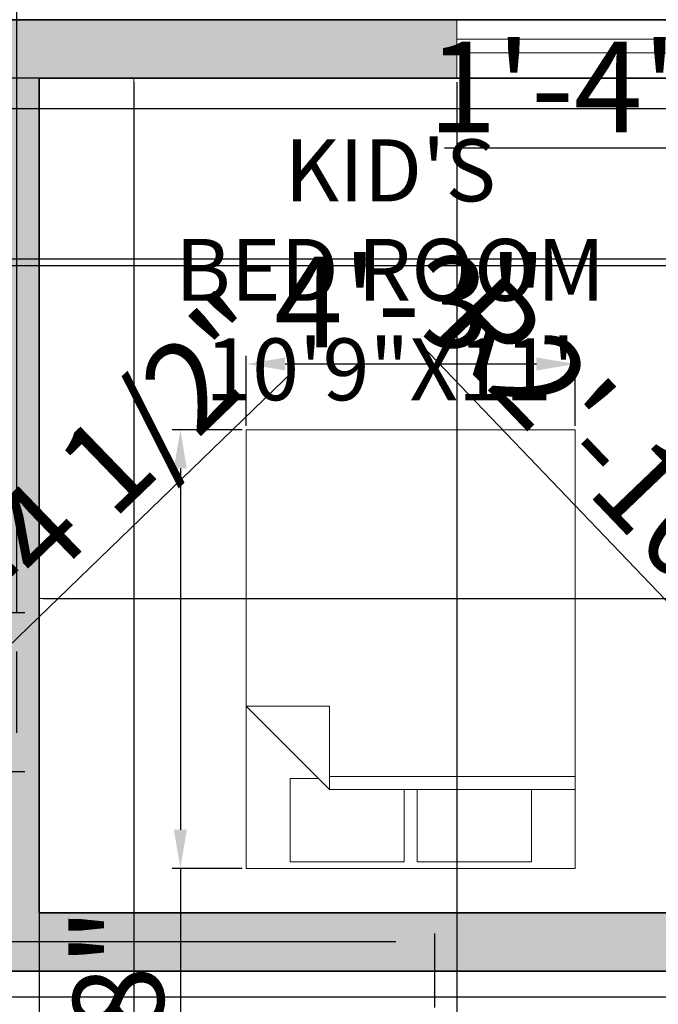
# Model space of a CAD drawing. Units: inches. Extents: x 2961 to 3748, y 1432 to 1961.
# Tile 5 of 9: x 3120 to 3219, y 1713 to 1865. Entities that reach past the tile are written whole.
import ezdxf
from ezdxf.enums import TextEntityAlignment as Align

# ---------------------------------------------------------------- set-up
doc = ezdxf.new("R2010")
doc.units = ezdxf.units.IN
for name, color, linetype, lineweight in [('A-ANNO-DIMS', 2, 'Continuous', 18), ('A-AREA-IDEN', 7, 'Continuous', 18), ('A-FURN', 8, 'Continuous', 18), ('A-FURN-FIXD', 9, 'Continuous', 20), ('A-GLAZ', 4, 'Continuous', 18), ('A-WALL', 7, 'Continuous', 35), ('A-WALL-PATT', 252, 'Continuous', 13)]:
    doc.layers.add(name, color=color, linetype=linetype, lineweight=lineweight)
doc.styles.get("Standard").update_dxf_attribs({"font": 'arial.ttf'})
doc.dimstyles.new('ISO-25', dxfattribs={"dimtxt": 14, "dimasz": 6, "dimexe": 1.25, "dimexo": 0.625, "dimtad": 1, "dimlunit": 3, "dimtxsty": 'Standard', "dimcen": 2.5, "dimadec": 0, "dimazin": 0, "dimtfac": 1, "dimtmove": 0, "dimatfit": 3, "dimfxl": 1, "dimarcsym": 0})

# ---------------------------------------------------------------- blocks, each defined once
blk = doc.blocks.new('Bed - Queen')
for p, q in [((0, -80.00003), (0, 0)), ((0, 0), (59.99999, 0)), ((59.99999, 0), (59.99999, -80.00003)), ((7.99999, -1.2), (28.79998, -1.2)), ((7.99999, -14.4), (7.99999, -1.2)), ((28.79998, -1.2), (28.79998, -14.4)), ((31.19999, -1.2), (51.99999, -1.2)), ((31.19999, -14.4), (31.19999, -1.2)), ((51.99999, -1.2), (51.99999, -16.4)), ((0, -14.4), (44.8, -14.4)), ((59.99999, -29.6), (44.8, -14.4)), ((44.8, -14.4), (44.8, -29.6)), ((44.8, -16.8), (0, -16.8)), ((51.99999, -16.4), (46.79936, -16.4)), ((44.8, -29.6), (59.99999, -29.6)), ((59.99999, -80.00003), (0, -80.00003))]:
    blk.add_line(p, q)
blk = doc.blocks.new('*D14')
at = {"layer": 'A-ANNO-DIMS', "color": 0, "lineweight": -2, "transparency": 16777216}
for p, q in [((3054.27, 1865.26), (3054.27, 1895.31)), ((3603.27, 1865.26), (3603.27, 1895.31)), ((3060.27, 1894.06), (3597.27, 1894.06))]:
    blk.add_line(p, q, dxfattribs=at)
at = {"layer": 'A-ANNO-DIMS', "color": 0, "transparency": 16777216}
for points in [[(3060.27, 1895.06), (3060.27, 1893.06), (3054.27, 1894.06)], [(3597.27, 1895.06), (3597.27, 1893.06), (3603.27, 1894.06)]]:
    blk.add_solid(points, dxfattribs=at)
at = {"layer": 'Defpoints', "color": 0, "transparency": 16777216}
for p in [(3603.27, 1894.06), (3054.27, 1864.64), (3603.27, 1864.64)]:
    blk.add_point(p, dxfattribs=at)
at = {"layer": 'A-ANNO-DIMS', "color": 0, "transparency": 16777216, "insert": (3328.77, 1901.84), "char_height": 14, "attachment_point": 5}
blk.add_mtext('45\'-9"', dxfattribs=at)
blk = doc.blocks.new('WIN-36IN')
for p, q in [((0, 6), (36, 6)), ((0, 3.9), (36, 3.9))]:
    blk.add_line(p, q)
blk.add_lwpolyline([(36, 9), (0, 9), (0, 0), (36, 0)], close=True)
blk = doc.blocks.new('*D24')
at = {"layer": 'A-ANNO-DIMS', "color": 0, "lineweight": -2, "transparency": 16777216}
for p, q in [((3154.63, 1801.29), (3143.84, 1801.29)), ((3145.09, 1795.29), (3145.09, 1739.5)), ((3154.63, 1733.5), (3143.84, 1733.5)), ((3145.09, 1733.5), (3145.09, 1644.01))]:
    blk.add_line(p, q, dxfattribs=at)
at = {"layer": 'A-ANNO-DIMS', "color": 0, "transparency": 16777216}
for points in [[(3144.09, 1795.29), (3146.09, 1795.29), (3145.09, 1801.29)], [(3144.09, 1739.5), (3146.09, 1739.5), (3145.09, 1733.5)]]:
    blk.add_solid(points, dxfattribs=at)
at = {"layer": 'Defpoints', "color": 0, "transparency": 16777216}
for p in [(3155.26, 1801.29), (3145.09, 1733.5), (3155.26, 1733.5)]:
    blk.add_point(p, dxfattribs=at)
at = {"layer": 'A-ANNO-DIMS', "color": 0, "transparency": 16777216, "insert": (3137.32, 1685.76), "char_height": 14, "attachment_point": 5, "rotation": 90}
blk.add_mtext('BED 5\'-8"', dxfattribs=at)
blk = doc.blocks.new('*D25')
at = {"layer": 'A-ANNO-DIMS', "color": 0, "lineweight": -2, "transparency": 16777216}
for p, q in [((3155.26, 1801.92), (3155.26, 1812.71)), ((3206.1, 1801.92), (3206.1, 1812.71)), ((3200.1, 1811.46), (3161.26, 1811.46))]:
    blk.add_line(p, q, dxfattribs=at)
at = {"layer": 'A-ANNO-DIMS', "color": 0, "transparency": 16777216}
for points in [[(3161.26, 1812.46), (3161.26, 1810.46), (3155.26, 1811.46)], [(3200.1, 1812.46), (3200.1, 1810.46), (3206.1, 1811.46)]]:
    blk.add_solid(points, dxfattribs=at)
at = {"layer": 'Defpoints', "color": 0, "transparency": 16777216}
for p in [(3155.26, 1811.46), (3155.26, 1801.29), (3206.1, 1801.29)]:
    blk.add_point(p, dxfattribs=at)
at = {"layer": 'A-ANNO-DIMS', "color": 0, "transparency": 16777216, "insert": (3180.68, 1819.24), "char_height": 14, "attachment_point": 5}
blk.add_mtext('4\'-3"', dxfattribs=at)
blk = doc.blocks.new('*D26')
at = {"layer": 'A-ANNO-DIMS', "color": 0, "lineweight": -2, "transparency": 16777216}
for p, q in [((3112.4, 1712.02), (3112.4, 1723.44)), ((3184.4, 1712.02), (3184.4, 1723.44)), ((3112.4, 1722.19), (2961.2, 1722.19)), ((3178.4, 1722.19), (3118.4, 1722.19))]:
    blk.add_line(p, q, dxfattribs=at)
at = {"layer": 'A-ANNO-DIMS', "color": 0, "transparency": 16777216}
for points in [[(3118.4, 1723.19), (3118.4, 1721.19), (3112.4, 1722.19)], [(3178.4, 1723.19), (3178.4, 1721.19), (3184.4, 1722.19)]]:
    blk.add_solid(points, dxfattribs=at)
at = {"layer": 'Defpoints', "color": 0, "transparency": 16777216}
for p in [(3112.4, 1722.19), (3112.4, 1711.39), (3184.4, 1711.39)]:
    blk.add_point(p, dxfattribs=at)
at = {"layer": 'A-ANNO-DIMS', "color": 0, "transparency": 16777216, "insert": (3033.8, 1730.06), "char_height": 14, "attachment_point": 5}
blk.add_mtext('SOFA 6\'-0" TYP.', dxfattribs=at)
blk = doc.blocks.new('*D28')
at = {"layer": 'A-ANNO-DIMS', "color": 0, "lineweight": -2, "transparency": 16777216}
for p, q in [((3253.06, 1631.67), (3253.06, 1776.5)), ((3245.67, 1631.67), (3254.31, 1631.67)), ((3253.06, 1584.22), (3253.06, 1625.67)), ((3245.67, 1578.22), (3254.31, 1578.22))]:
    blk.add_line(p, q, dxfattribs=at)
at = {"layer": 'A-ANNO-DIMS', "color": 0, "transparency": 16777216}
for points in [[(3252.06, 1625.67), (3254.06, 1625.67), (3253.06, 1631.67)], [(3252.06, 1584.22), (3254.06, 1584.22), (3253.06, 1578.22)]]:
    blk.add_solid(points, dxfattribs=at)
at = {"layer": 'Defpoints', "color": 0, "transparency": 16777216}
for p in [(3245.04, 1631.67), (3253.06, 1631.67), (3245.04, 1578.22)]:
    blk.add_point(p, dxfattribs=at)
at = {"layer": 'A-ANNO-DIMS', "color": 0, "transparency": 16777216, "insert": (3245.19, 1707.08), "char_height": 14, "attachment_point": 5, "rotation": 90}
blk.add_mtext('TABLE 4\'-5 1/2"', dxfattribs=at)
blk = doc.blocks.new('*D31')
at = {"layer": 'A-ANNO-DIMS', "color": 0, "lineweight": -2, "transparency": 16777216}
for p, q in [((3229.02, 1840.61), (3229.02, 1846.04)), ((3245.04, 1840.61), (3245.04, 1846.04)), ((3229.02, 1844.79), (3185.88, 1844.79)), ((3239.04, 1844.79), (3235.02, 1844.79))]:
    blk.add_line(p, q, dxfattribs=at)
at = {"layer": 'A-ANNO-DIMS', "color": 0, "transparency": 16777216}
for points in [[(3235.02, 1845.79), (3235.02, 1843.79), (3229.02, 1844.79)], [(3239.04, 1845.79), (3239.04, 1843.79), (3245.04, 1844.79)]]:
    blk.add_solid(points, dxfattribs=at)
at = {"layer": 'Defpoints', "color": 0, "transparency": 16777216}
for p in [(3229.02, 1844.79), (3229.02, 1839.99), (3245.04, 1839.99)]:
    blk.add_point(p, dxfattribs=at)
at = {"layer": 'A-ANNO-DIMS', "color": 0, "transparency": 16777216, "insert": (3204.45, 1852.45), "char_height": 14, "attachment_point": 5}
blk.add_mtext('1\'-4"', dxfattribs=at)
blk = doc.blocks.new('*D46')
at = {"layer": 'A-ANNO-DIMS', "color": 0, "lineweight": -2, "transparency": 16777216}
for p, q in [((3119.82, 1773.04), (3119.82, 1913.63)), ((3116.76, 1773.04), (3121.07, 1773.04)), ((3119.82, 1754.49), (3119.82, 1767.04)), ((3116.76, 1748.49), (3121.07, 1748.49))]:
    blk.add_line(p, q, dxfattribs=at)
at = {"layer": 'A-ANNO-DIMS', "color": 0, "transparency": 16777216}
for points in [[(3118.82, 1767.04), (3120.82, 1767.04), (3119.82, 1773.04)], [(3118.82, 1754.49), (3120.82, 1754.49), (3119.82, 1748.49)]]:
    blk.add_solid(points, dxfattribs=at)
at = {"layer": 'Defpoints', "color": 0, "transparency": 16777216}
for p in [(3116.13, 1773.04), (3119.82, 1773.04), (3116.13, 1748.49)]:
    blk.add_point(p, dxfattribs=at)
at = {"layer": 'A-ANNO-DIMS', "color": 0, "transparency": 16777216, "insert": (3111.95, 1846.34), "char_height": 14, "attachment_point": 5, "rotation": 90}
blk.add_mtext('BASIN 2\'-0 1/2"', dxfattribs=at)
blk = doc.blocks.new('*D53')
at = {"layer": 'A-ANNO-DIMS', "color": 0, "lineweight": -2, "transparency": 16777216}
for p, q in [((3123.27, 1855.01), (3123.27, 1473.94)), ((3187.8, 1855.01), (3187.8, 1473.94)), ((3129.27, 1475.19), (3181.8, 1475.19)), ((3187.8, 1475.19), (3264.89, 1475.19))]:
    blk.add_line(p, q, dxfattribs=at)
at = {"layer": 'A-ANNO-DIMS', "color": 0, "transparency": 16777216}
for points in [[(3129.27, 1476.19), (3129.27, 1474.19), (3123.27, 1475.19)], [(3181.8, 1476.19), (3181.8, 1474.19), (3187.8, 1475.19)]]:
    blk.add_solid(points, dxfattribs=at)
at = {"layer": 'Defpoints', "color": 0, "transparency": 16777216}
for p in [(3123.27, 1855.64), (3187.8, 1855.64), (3187.8, 1475.19)]:
    blk.add_point(p, dxfattribs=at)
at = {"layer": 'A-ANNO-DIMS', "color": 0, "transparency": 16777216, "insert": (3229.35, 1483.05), "char_height": 14, "attachment_point": 5}
blk.add_mtext('5\'-4 1/2"', dxfattribs=at)
blk = doc.blocks.new('*D64')
at = {"layer": 'A-ANNO-DIMS', "color": 0, "lineweight": -2, "transparency": 16777216}
for p, q in [((3509.64, 1855.64), (3023.57, 1855.64)), ((3024.82, 1849.64), (3024.82, 1833.64)), ((3509.64, 1827.64), (3023.57, 1827.64)), ((3024.82, 1827.64), (3024.82, 1782.93))]:
    blk.add_line(p, q, dxfattribs=at)
at = {"layer": 'A-ANNO-DIMS', "color": 0, "transparency": 16777216}
for points in [[(3023.82, 1849.64), (3025.82, 1849.64), (3024.82, 1855.64)], [(3023.82, 1833.64), (3025.82, 1833.64), (3024.82, 1827.64)]]:
    blk.add_solid(points, dxfattribs=at)
at = {"layer": 'Defpoints', "color": 0, "transparency": 16777216}
for p in [(3510.27, 1855.64), (3024.82, 1827.64), (3510.27, 1827.64)]:
    blk.add_point(p, dxfattribs=at)
at = {"layer": 'A-ANNO-DIMS', "color": 0, "transparency": 16777216, "insert": (3017.16, 1802.29), "char_height": 14, "attachment_point": 5, "rotation": 90}
blk.add_mtext('2\'-4"', dxfattribs=at)
blk = doc.blocks.new('*D73')
at = {"layer": 'A-ANNO-DIMS', "color": 0, "lineweight": -2, "transparency": 16777216}
for p, q in [((3069.27, 1717.01), (3069.27, 1473.94)), ((3103.27, 1717.01), (3103.27, 1473.94)), ((3075.27, 1475.19), (3097.27, 1475.19)), ((3103.27, 1475.19), (3158.85, 1475.19))]:
    blk.add_line(p, q, dxfattribs=at)
at = {"layer": 'A-ANNO-DIMS', "color": 0, "transparency": 16777216}
for points in [[(3075.27, 1476.19), (3075.27, 1474.19), (3069.27, 1475.19)], [(3097.27, 1476.19), (3097.27, 1474.19), (3103.27, 1475.19)]]:
    blk.add_solid(points, dxfattribs=at)
at = {"layer": 'Defpoints', "color": 0, "transparency": 16777216}
for p in [(3069.27, 1717.64), (3103.27, 1717.64), (3103.27, 1475.19)]:
    blk.add_point(p, dxfattribs=at)
at = {"layer": 'A-ANNO-DIMS', "color": 0, "transparency": 16777216, "insert": (3134.06, 1482.96), "char_height": 14, "attachment_point": 5}
blk.add_mtext('2\'-10"', dxfattribs=at)
blk = doc.blocks.new('*D74')
at = {"layer": 'A-ANNO-DIMS', "color": 0, "lineweight": -2, "transparency": 16777216}
for p, q in [((3117.27, 1726.01), (3117.27, 1473.94)), ((3103.27, 1717.01), (3103.27, 1473.94)), ((3109.27, 1475.19), (3111.27, 1475.19)), ((3117.27, 1475.19), (3160.41, 1475.19))]:
    blk.add_line(p, q, dxfattribs=at)
at = {"layer": 'A-ANNO-DIMS', "color": 0, "transparency": 16777216}
for points in [[(3109.27, 1476.19), (3109.27, 1474.19), (3103.27, 1475.19)], [(3111.27, 1476.19), (3111.27, 1474.19), (3117.27, 1475.19)]]:
    blk.add_solid(points, dxfattribs=at)
at = {"layer": 'Defpoints', "color": 0, "transparency": 16777216}
for p in [(3117.27, 1726.64), (3103.27, 1717.64), (3117.27, 1475.19)]:
    blk.add_point(p, dxfattribs=at)
at = {"layer": 'A-ANNO-DIMS', "color": 0, "transparency": 16777216, "insert": (3141.84, 1482.84), "char_height": 14, "attachment_point": 5}
blk.add_mtext('1\'-2"', dxfattribs=at)
blk = doc.blocks.new('*D75')
at = {"layer": 'A-ANNO-DIMS', "color": 0, "lineweight": -2, "transparency": 16777216}
for p, q in [((3024.82, 1723.64), (3024.82, 1729.64)), ((3254.64, 1717.64), (3023.57, 1717.64)), ((3024.82, 1717.64), (3024.82, 1713.64)), ((3254.64, 1713.64), (3023.57, 1713.64)), ((3024.82, 1707.64), (3024.82, 1663.17))]:
    blk.add_line(p, q, dxfattribs=at)
at = {"layer": 'A-ANNO-DIMS', "color": 0, "transparency": 16777216}
for points in [[(3023.82, 1723.64), (3025.82, 1723.64), (3024.82, 1717.64)], [(3023.82, 1707.64), (3025.82, 1707.64), (3024.82, 1713.64)]]:
    blk.add_solid(points, dxfattribs=at)
at = {"layer": 'Defpoints', "color": 0, "transparency": 16777216}
for p in [(3255.27, 1717.64), (3024.82, 1713.64), (3255.27, 1713.64)]:
    blk.add_point(p, dxfattribs=at)
at = {"layer": 'A-ANNO-DIMS', "color": 0, "transparency": 16777216, "insert": (3017.04, 1682.41), "char_height": 14, "attachment_point": 5, "rotation": 90}
blk.add_mtext('0\'-4"', dxfattribs=at)
blk = doc.blocks.new('*D82')
at = {"layer": 'A-ANNO-DIMS', "color": 0, "lineweight": -2, "transparency": 16777216}
for p, q in [((3063.27, 1542.49), (3063.27, 1933.63)), ((3069.27, 1932.38), (3078.82, 1932.38)), ((3084.82, 1542.49), (3084.82, 1933.63)), ((3084.82, 1932.38), (3160.59, 1932.38))]:
    blk.add_line(p, q, dxfattribs=at)
at = {"layer": 'A-ANNO-DIMS', "color": 0, "transparency": 16777216}
for points in [[(3069.27, 1933.38), (3069.27, 1931.38), (3063.27, 1932.38)], [(3078.82, 1933.38), (3078.82, 1931.38), (3084.82, 1932.38)]]:
    blk.add_solid(points, dxfattribs=at)
at = {"layer": 'Defpoints', "color": 0, "transparency": 16777216}
for p in [(3084.82, 1932.38), (3063.27, 1541.87), (3084.82, 1541.87)]:
    blk.add_point(p, dxfattribs=at)
at = {"layer": 'A-ANNO-DIMS', "color": 0, "transparency": 16777216, "insert": (3125.71, 1940.24), "char_height": 14, "attachment_point": 5}
blk.add_mtext('1\'-9 1/2"', dxfattribs=at)
blk = doc.blocks.new('*D83')
at = {"layer": 'A-ANNO-DIMS', "color": 0, "lineweight": -2, "transparency": 16777216}
for p, q in [((3123.89, 1855.64), (3633.97, 1855.64)), ((3632.72, 1781.22), (3632.72, 1849.64)), ((3123.89, 1775.22), (3633.97, 1775.22))]:
    blk.add_line(p, q, dxfattribs=at)
at = {"layer": 'A-ANNO-DIMS', "color": 0, "transparency": 16777216}
for points in [[(3631.72, 1849.64), (3633.72, 1849.64), (3632.72, 1855.64)], [(3631.72, 1781.22), (3633.72, 1781.22), (3632.72, 1775.22)]]:
    blk.add_solid(points, dxfattribs=at)
at = {"layer": 'Defpoints', "color": 0, "transparency": 16777216}
for p in [(3123.27, 1855.64), (3632.72, 1855.64), (3123.27, 1775.22)]:
    blk.add_point(p, dxfattribs=at)
at = {"layer": 'A-ANNO-DIMS', "color": 0, "transparency": 16777216, "insert": (3624.85, 1815.43), "char_height": 14, "attachment_point": 5, "rotation": 90}
blk.add_mtext('6\'-8 1/2"', dxfattribs=at)
blk = doc.blocks.new('*D84')
at = {"layer": 'A-ANNO-DIMS', "color": 0, "lineweight": -2, "transparency": 16777216}
for p, q in [((3123.27, 1855.01), (3123.27, 1473.94)), ((3137.88, 1855.01), (3137.88, 1473.94)), ((3129.27, 1475.19), (3131.88, 1475.19)), ((3137.88, 1475.19), (3213.65, 1475.19))]:
    blk.add_line(p, q, dxfattribs=at)
at = {"layer": 'A-ANNO-DIMS', "color": 0, "transparency": 16777216}
for points in [[(3129.27, 1476.19), (3129.27, 1474.19), (3123.27, 1475.19)], [(3131.88, 1476.19), (3131.88, 1474.19), (3137.88, 1475.19)]]:
    blk.add_solid(points, dxfattribs=at)
at = {"layer": 'Defpoints', "color": 0, "transparency": 16777216}
for p in [(3123.27, 1855.64), (3137.88, 1855.64), (3137.88, 1475.19)]:
    blk.add_point(p, dxfattribs=at)
at = {"layer": 'A-ANNO-DIMS', "color": 0, "transparency": 16777216, "insert": (3178.76, 1483.05), "char_height": 14, "attachment_point": 5}
blk.add_mtext('1\'-2 1/2"', dxfattribs=at)
blk = doc.blocks.new('*D86')
at = {"layer": 'A-ANNO-DIMS', "color": 0, "lineweight": -2, "transparency": 16777216}
for p, q in [((3091.52, 1850.93), (3633.97, 1850.93)), ((3632.72, 1844.93), (3632.72, 1832.66)), ((3082.42, 1826.66), (3633.97, 1826.66)), ((3632.72, 1826.66), (3632.72, 1749.34))]:
    blk.add_line(p, q, dxfattribs=at)
at = {"layer": 'A-ANNO-DIMS', "color": 0, "transparency": 16777216}
for points in [[(3631.72, 1844.93), (3633.72, 1844.93), (3632.72, 1850.93)], [(3631.72, 1832.66), (3633.72, 1832.66), (3632.72, 1826.66)]]:
    blk.add_solid(points, dxfattribs=at)
at = {"layer": 'Defpoints', "color": 0, "transparency": 16777216}
for p in [(3090.9, 1850.93), (3081.8, 1826.66), (3632.72, 1826.66)]:
    blk.add_point(p, dxfattribs=at)
at = {"layer": 'A-ANNO-DIMS', "color": 0, "transparency": 16777216, "insert": (3624.85, 1785), "char_height": 14, "attachment_point": 5, "rotation": 90}
blk.add_mtext('2\'-0 1/2"', dxfattribs=at)
blk = doc.blocks.new('*D94')
at = {"layer": 'A-ANNO-DIMS', "color": 0, "lineweight": -2, "transparency": 16777216}
for p, q in [((3182.5, 1814.2), (3230.05, 1764.56)), ((3257.56, 1735.84), (3234.2, 1760.22))]:
    blk.add_line(p, q, dxfattribs=at)
at = {"layer": 'A-ANNO-DIMS', "color": 0, "transparency": 16777216}
blk.add_solid([(3230.78, 1765.25), (3229.33, 1763.87), (3234.2, 1760.22)], dxfattribs=at)
at = {"layer": 'Defpoints', "color": 0, "transparency": 16777216}
for p in [(3234.2, 1760.22), (3257.56, 1735.84)]:
    blk.add_point(p, dxfattribs=at)
at = {"layer": 'A-ANNO-DIMS', "color": 0, "transparency": 16777216, "insert": (3209.82, 1796.92), "char_height": 14, "attachment_point": 5, "rotation": 313.7658}
blk.add_mtext('R2\'-10"', dxfattribs=at)
blk = doc.blocks.new('*D95')
at = {"layer": 'A-ANNO-DIMS', "color": 0, "lineweight": -2, "transparency": 16777216}
for p, q in [((3162.66, 1810.5), (3097.6, 1747.61)), ((3072.77, 1723.61), (3093.28, 1743.44))]:
    blk.add_line(p, q, dxfattribs=at)
at = {"layer": 'A-ANNO-DIMS', "color": 0, "transparency": 16777216}
blk.add_solid([(3096.9, 1748.33), (3098.29, 1746.89), (3093.28, 1743.44)], dxfattribs=at)
at = {"layer": 'Defpoints', "color": 0, "transparency": 16777216}
for p in [(3093.28, 1743.44), (3072.77, 1723.61)]:
    blk.add_point(p, dxfattribs=at)
at = {"layer": 'A-ANNO-DIMS', "color": 0, "transparency": 16777216, "insert": (3126.82, 1786.79), "char_height": 14, "attachment_point": 5, "rotation": 44.0296}
blk.add_mtext('R2\'-4 1/2"', dxfattribs=at)

msp = doc.modelspace()

# ---------------------------------------------------------------- hatches: boundary and pattern name
at = {"layer": 'A-WALL-PATT'}
h = msp.add_hatch(color=256, dxfattribs=at)
h.set_gradient(color1=(41, 49, 137), color2=(41, 49, 137), tint=1)
h.paths.add_polyline_path([(3255.267, 1671.639), (3255.267, 1513.639), (3251.267, 1513.639), (3251.267, 1504.639), (3268.267, 1504.639), (3268.267, 1513.639), (3264.267, 1513.639), (3264.267, 1671.639), (3259.767, 1671.639)])
h.paths.add_polyline_path([(3063.267, 1513.639), (3063.267, 1677.639), (3054.267, 1677.639), (3054.267, 1504.639), (3215.267, 1504.639), (3215.267, 1513.639)])
h.paths.add_polyline_path([(3304.267, 1513.639), (3304.267, 1504.639), (3456.267, 1504.639), (3456.267, 1513.639), (3390.267, 1513.639), (3390.267, 1605.639), (3384.267, 1605.639), (3384.267, 1513.639)])
h.paths.add_polyline_path([(3510.267, 1605.639), (3510.267, 1513.639), (3492.267, 1513.639), (3492.267, 1504.639), (3546.267, 1504.639), (3546.267, 1513.639), (3519.267, 1513.639), (3519.267, 1605.639)])
h.paths.add_polyline_path([(3340.267, 1654.639), (3340.267, 1645.639), (3510.267, 1645.639), (3510.267, 1641.639), (3519.267, 1641.639), (3519.267, 1658.639), (3510.267, 1658.639), (3510.267, 1654.639)])
h.paths.add_polyline_path([(3223.801, 1864.639), (3223.801, 1855.639), (3255.267, 1855.639), (3255.267, 1772.534), (3264.267, 1772.534), (3264.267, 1855.639), (3303.267, 1855.639), (3303.267, 1864.639)])
h.paths.add_polyline_path([(3339.267, 1864.639), (3339.267, 1855.639), (3435.267, 1855.639), (3435.267, 1864.639)])
h.paths.add_polyline_path([(3471.267, 1864.639), (3471.267, 1855.639), (3510.267, 1855.639), (3510.267, 1827.639), (3519.267, 1827.639), (3519.267, 1864.639)])
h.paths.add_polyline_path([(3510.267, 1767.639), (3510.267, 1739.639), (3519.267, 1739.639), (3519.267, 1767.639)])
h.paths.add_polyline_path([(3123.267, 1726.639), (3123.267, 1855.639), (3187.801, 1855.639), (3187.801, 1864.639), (3054.267, 1864.639), (3054.267, 1837.201), (3063.267, 1837.201), (3063.267, 1855.639), (3117.267, 1855.639), (3117.267, 1726.639), (3103.267, 1726.639), (3103.267, 1717.639), (3255.267, 1717.639), (3255.267, 1713.639), (3264.267, 1713.639), (3264.267, 1730.534), (3255.267, 1730.639), (3255.267, 1726.639)])
h.paths.add_polyline_path([(3597.267, 1654.639), (3597.267, 1513.639), (3570.267, 1513.639), (3570.267, 1504.639), (3603.267, 1504.639), (3603.267, 1654.639)])
h.paths.add_polyline_path([(3054.267, 1813.201), (3054.267, 1713.639), (3063.267, 1713.639), (3063.267, 1717.639), (3069.267, 1717.639), (3069.267, 1726.639), (3063.267, 1726.639), (3063.267, 1813.201)], flags=17)

# ---------------------------------------------------------------- linework, layer by layer
at = {"layer": 'A-FURN-FIXD'}
msp.add_lwpolyline([(3123.267, 1775.22), (3123.267, 1855.639), (3137.877, 1855.639), (3137.877, 1775.22)], close=True, dxfattribs=at)
at = {"layer": 'A-WALL'}
for p, q in [((3054.267, 1864.639), (3519.267, 1864.639)), ((3123.267, 1726.639), (3123.267, 1855.639)), ((3255.267, 1855.639), (3123.267, 1855.639)), ((3255.267, 1726.639), (3123.267, 1726.639)), ((3255.267, 1717.639), (3063.267, 1717.639))]:
    msp.add_line(p, q, dxfattribs=at)

# ---------------------------------------------------------------- block references
at = {"layer": 'A-FURN', "xscale": 0.8473786619107851, "yscale": 0.8473786619107851, "zscale": 0.8473786619107851, "rotation": 180}
msp.add_blockref('Bed - Queen', (3206.1, 1733.502), dxfattribs=at)
at = {"layer": 'A-GLAZ'}
msp.add_blockref('WIN-36IN', (3187.801, 1855.639), dxfattribs=at)

# ---------------------------------------------------------------- texts
at = {"layer": 'A-AREA-IDEN'}
for s, p in [("KID'S", (3177.513, 1836.597)), ('BED ROOM', (3177.513, 1821.223)), ('10\'9"X11\'', (3177.513, 1805.848))]:
    msp.add_text(s, height=9.5707, dxfattribs=at).set_placement(p, align=Align.CENTER)

# ---------------------------------------------------------------- dimensions: what is measured, and where the dimension line sits
at = {"layer": 'A-ANNO-DIMS'}
for base, p1, p2, override, picture, middle in [((3084.825, 1932.38), (3063.267, 1541.867), (3084.825, 1541.867), {"dimdec": 1, "dimlfac": 1, "dimrnd": 0, "dimzin": 1, "dimdsep": 46, "dimlunit": 4, "dimfrac": 2}, '*D82', (3125.71, 1940.244)), ((3603.267, 1894.063), (3054.267, 1864.639), (3603.267, 1864.639), {"dimclrd": 0, "dimclre": 0, "dimclrt": 0}, '*D14', (3328.767, 1901.836)), ((3187.801, 1475.189), (3123.267, 1855.639), (3187.801, 1855.639), {"dimdec": 1, "dimlfac": 1, "dimrnd": 0, "dimzin": 1, "dimdsep": 46, "dimlunit": 4, "dimfrac": 2}, '*D53', (3229.345, 1483.052)), ((3137.877, 1475.189), (3123.267, 1855.639), (3137.877, 1855.639), {"dimdec": 1, "dimlfac": 1, "dimrnd": 0, "dimzin": 1, "dimdsep": 46, "dimlunit": 4, "dimfrac": 2}, '*D84', (3178.762, 1483.052)), ((3117.267, 1475.189), (3103.267, 1717.639), (3117.267, 1726.639), {"dimdec": 1, "dimlfac": 1, "dimrnd": 0, "dimzin": 1, "dimdsep": 46, "dimlunit": 4, "dimfrac": 2}, '*D74', (3141.841, 1482.842)), ((3103.267, 1475.189), (3069.267, 1717.639), (3103.267, 1717.639), {"dimdec": 1, "dimlfac": 1, "dimrnd": 0, "dimzin": 1, "dimdsep": 46, "dimlunit": 4, "dimfrac": 2}, '*D73', (3134.058, 1482.962))]:
    dim = msp.add_linear_dim(base=base, p1=p1, p2=p2, dimstyle='ISO-25', override=override, dxfattribs=at)
    dim.commit()
    dim.dimension.update_dxf_attribs({"geometry": picture, "text_midpoint": middle})
for base, p1, p2, angle, text, picture, middle in [((3119.818, 1773.04), (3116.135, 1748.489), (3116.135, 1773.04), 90, 'BASIN <>', '*D46', (3111.954, 1846.336)), ((3145.088, 1733.502), (3155.257, 1801.293), (3155.257, 1733.502), 270, 'BED <>', '*D24', (3137.315, 1685.756)), ((3253.058, 1631.667), (3245.042, 1578.224), (3245.042, 1631.667), 90, 'TABLE <>', '*D28', (3245.195, 1707.084)), ((3112.401, 1722.191), (3184.401, 1711.391), (3112.401, 1711.391), 180, 'SOFA <> TYP.', '*D26', (3033.799, 1730.06))]:
    dim = msp.add_linear_dim(base=base, p1=p1, p2=p2, angle=angle, text=text, dimstyle='ISO-25', override={"dimdec": 1, "dimlfac": 1, "dimrnd": 0, "dimzin": 1, "dimdsep": 46, "dimlunit": 4, "dimfrac": 2}, dxfattribs=at)
    dim.commit()
    dim.dimension.update_dxf_attribs({"geometry": picture, "text_midpoint": middle})
for base, p1, p2, angle, picture, middle in [((3229.024, 1844.793), (3245.042, 1839.987), (3229.024, 1839.987), 180, '*D31', (3204.45, 1852.446)), ((3024.817, 1827.639), (3510.267, 1855.639), (3510.267, 1827.639), 90, '*D64', (3017.163, 1802.287)), ((3632.717, 1855.639), (3123.267, 1775.22), (3123.267, 1855.639), 90, '*D83', (3624.853, 1815.429)), ((3632.717, 1826.664), (3090.897, 1850.93), (3081.797, 1826.664), 90, '*D86', (3624.853, 1785)), ((3155.257, 1811.461), (3206.1, 1801.293), (3155.257, 1801.293), 180, '*D25', (3180.678, 1819.239)), ((3024.817, 1713.639), (3255.267, 1717.639), (3255.267, 1713.639), 90, '*D75', (3017.044, 1682.406))]:
    dim = msp.add_linear_dim(base=base, p1=p1, p2=p2, angle=angle, dimstyle='ISO-25', override={"dimdec": 1, "dimlfac": 1, "dimrnd": 0, "dimzin": 1, "dimdsep": 46, "dimlunit": 4, "dimfrac": 2}, dxfattribs=at)
    dim.commit()
    dim.dimension.update_dxf_attribs({"geometry": picture, "text_midpoint": middle})
for center, mpoint, picture, middle in [((3257.563, 1735.836), (3234.204, 1760.224), '*D94', (3209.817, 1796.922)), ((3072.767, 1723.605), (3093.285, 1743.44), '*D95', (3126.819, 1786.794))]:
    dim = msp.add_radius_dim(center=center, mpoint=mpoint, dimstyle='ISO-25', override={"dimdec": 1, "dimlfac": 1, "dimrnd": 0, "dimzin": 1, "dimdsep": 46, "dimlunit": 4, "dimfrac": 2}, dxfattribs=at)
    dim.commit()
    dim.dimension.update_dxf_attribs({"geometry": picture, "text_midpoint": middle})

doc.saveas('drawing.dxf')
